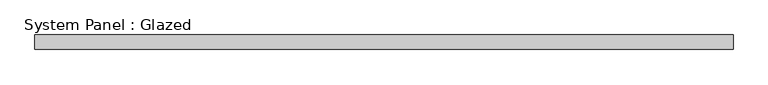
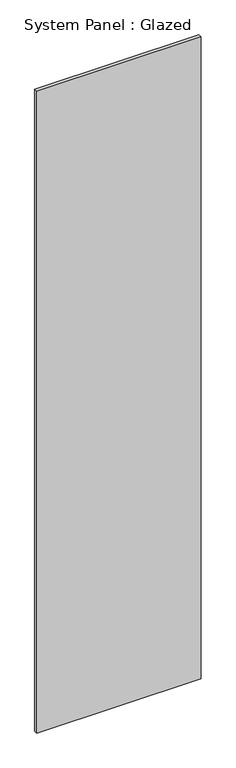
"""IFC4 building model written with IfcOpenShell, lengths in millimetres: plate geometry, System Panel : Glazed."""

from ifc_helpers import new_model, si_unit, origin, origin_with_axes, place, context, project, spatial, polyline, outline, extrude, source, transform, mapped, element, save


def system_panel_glazed_8799d416(model_context):
    return source(origin(), model_context, "Body", "SweptSolid", [
        extrude(outline(polyline([(600.0, 24.5), (-600.0, 24.5), (-600.0, 49.5), (600.0, 49.5), (600.0, 24.5)])), origin_with_axes(), (0.0, 0.0, 1.0), 4950.0),
    ])


if __name__ == "__main__":
    model = new_model("IFC4")
    model_context = context("Model", 3, world=origin())
    ifc_project = project(units=[si_unit("LENGTHUNIT", "METRE", prefix="MILLI")], contexts=[model_context])
    site = spatial("IfcSite", under=ifc_project)
    building = spatial("IfcBuilding", under=site)
    placement = place(None, origin())
    system_panel_glazed_shape = system_panel_glazed_8799d416(model_context)
    element("IfcPlate", 1, ObjectType="System Panel : Glazed", at=placement, inside=building, context=model_context, shape_type="MappedRepresentation", body=[
        mapped(system_panel_glazed_shape, transform((0.0, 0.0, 0.0), x_axis=(1.0, 0.0, 0.0), y_axis=(0.0, 1.0, 0.0), z_axis=(0.0, 0.0, 1.0))),
    ])
    save(model, "model.ifc")

# Revit data of these elements
# Element 1 (IfcPlate, "System Panel : Glazed")
#   Materials on its faces: "Glass"
# Materials
#   "Glass": class "Glass", colour RGB 218 227 224, transparency 0.85, Description = "Soda Lime Glass", Cost = 0
